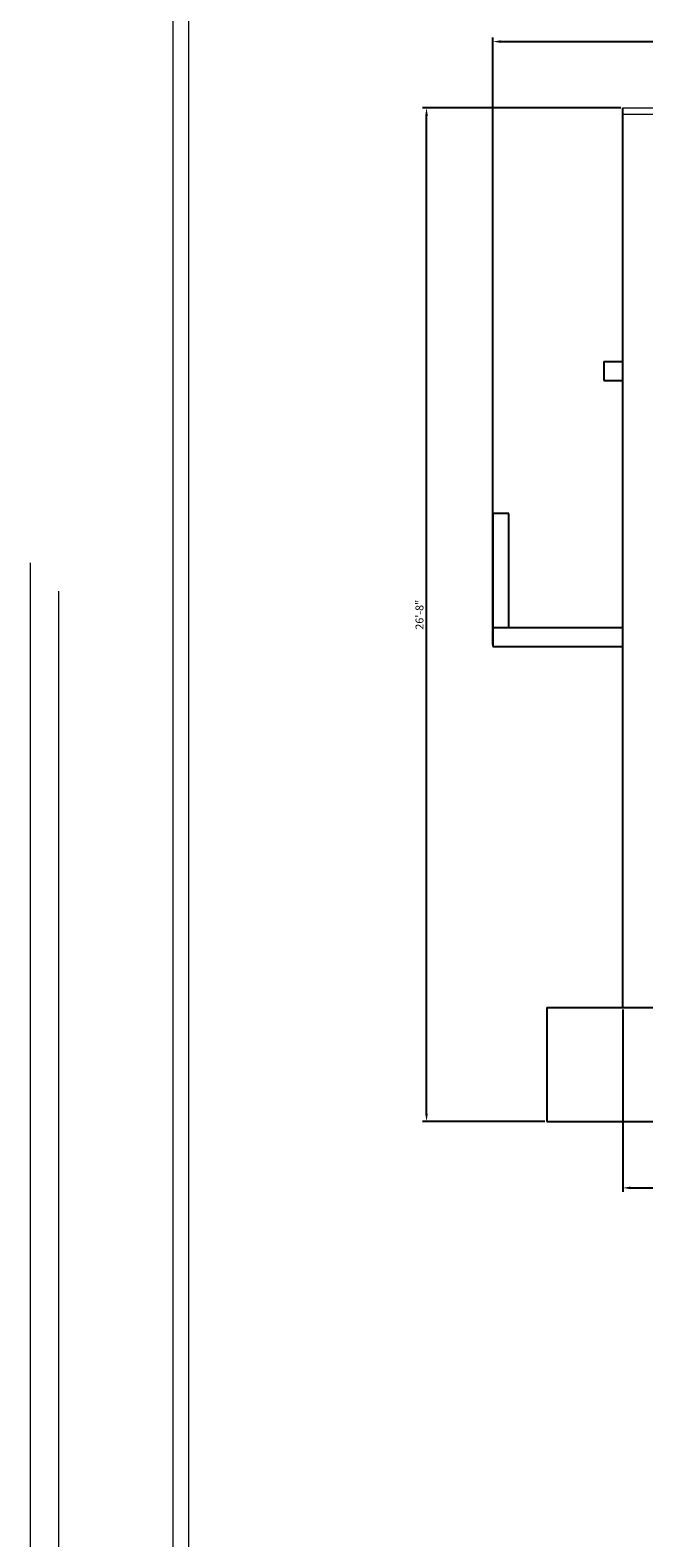
# Model space of a CAD drawing. Units: inches. Extents: x 2443635 to 2446153, y 1826255 to 1827341.
# Tile 15 of 16: x 2445578 to 2445772, y 1826731 to 1827207. Entities that reach past the tile are written whole.
import ezdxf

# ---------------------------------------------------------------- set-up
doc = ezdxf.new("R2010")
doc.units = ezdxf.units.IN
for name, color, linetype, lineweight in [('A-DIMS', 1, 'Continuous', 18), ('A-ELEV', 7, 'Continuous', 25), ('A-ELEV-RAIL', 9, 'Continuous', 18), ('A-REFR', 8, 'Continuous', 13)]:
    doc.layers.add(name, color=color, linetype=linetype, lineweight=lineweight)
doc.styles.get("Standard").update_dxf_attribs({"font": 'arial.ttf'})
doc.dimstyles.new('ISO-25', dxfattribs={"dimtxt": 2.5, "dimasz": 2.5, "dimexe": 1.25, "dimexo": 0.625, "dimtad": 1, "dimlunit": 4, "dimtxsty": 'Standard', "dimcen": 2.5, "dimadec": 0, "dimazin": 0, "dimtfac": 1, "dimtmove": 0, "dimatfit": 3, "dimfxl": 1, "dimarcsym": 0})

# ---------------------------------------------------------------- blocks, each defined once
blk = doc.blocks.new('*D107')
at = {"layer": 'A-DIMS', "color": 0, "lineweight": -2, "transparency": 16777216}
for p, q in [((2445724.56, 1827013.33), (2445724.56, 1827204.9)), ((2446130.56, 1827013.33), (2446130.56, 1827204.9)), ((2445727.06, 1827203.65), (2446128.06, 1827203.65))]:
    blk.add_line(p, q, dxfattribs=at)
at = {"layer": 'A-DIMS', "color": 0, "transparency": 16777216}
for points in [[(2445727.06, 1827204.07), (2445727.06, 1827203.23), (2445724.56, 1827203.65)], [(2446128.06, 1827204.07), (2446128.06, 1827203.23), (2446130.56, 1827203.65)]]:
    blk.add_solid(points, dxfattribs=at)
at = {"layer": 'Defpoints', "color": 0, "transparency": 16777216}
for p in [(2446130.56, 1827203.65), (2445724.56, 1827012.7), (2446130.56, 1827012.7)]:
    blk.add_point(p, dxfattribs=at)
at = {"layer": 'A-DIMS', "color": 0, "transparency": 16777216, "insert": (2445927.56, 1827205.55), "char_height": 2.5, "attachment_point": 5}
blk.add_mtext('33\'-10"', dxfattribs=at)
blk = doc.blocks.new('*D108')
at = {"layer": 'A-DIMS', "color": 0, "lineweight": -2, "transparency": 16777216}
for p, q in [((2445764.93, 1827182.7), (2445702.36, 1827182.7)), ((2445703.61, 1826865.2), (2445703.61, 1827180.2)), ((2445740.93, 1826862.7), (2445702.36, 1826862.7))]:
    blk.add_line(p, q, dxfattribs=at)
at = {"layer": 'A-DIMS', "color": 0, "transparency": 16777216}
for points in [[(2445703.19, 1827180.2), (2445704.03, 1827180.2), (2445703.61, 1827182.7)], [(2445703.19, 1826865.2), (2445704.03, 1826865.2), (2445703.61, 1826862.7)]]:
    blk.add_solid(points, dxfattribs=at)
at = {"layer": 'Defpoints', "color": 0, "transparency": 16777216}
for p in [(2445703.61, 1827182.7), (2445765.56, 1827182.7), (2445741.56, 1826862.7)]:
    blk.add_point(p, dxfattribs=at)
at = {"layer": 'A-DIMS', "color": 0, "transparency": 16777216, "insert": (2445701.71, 1827022.7), "char_height": 2.5, "attachment_point": 5, "rotation": 90}
blk.add_mtext('26\'-8"', dxfattribs=at)
blk = doc.blocks.new('*D109')
at = {"layer": 'A-DIMS', "color": 0, "lineweight": -2, "transparency": 16777216}
for p, q in [((2445765.56, 1826898.08), (2445765.56, 1826840.5)), ((2445906.56, 1826898.08), (2445906.56, 1826840.5)), ((2445768.06, 1826841.75), (2445904.06, 1826841.75))]:
    blk.add_line(p, q, dxfattribs=at)
at = {"layer": 'A-DIMS', "color": 0, "transparency": 16777216}
for points in [[(2445768.06, 1826842.17), (2445768.06, 1826841.33), (2445765.56, 1826841.75)], [(2445904.06, 1826842.17), (2445904.06, 1826841.33), (2445906.56, 1826841.75)]]:
    blk.add_solid(points, dxfattribs=at)
at = {"layer": 'Defpoints', "color": 0, "transparency": 16777216}
for p in [(2445765.56, 1826898.7), (2445906.56, 1826898.7), (2445906.56, 1826841.75)]:
    blk.add_point(p, dxfattribs=at)
at = {"layer": 'A-DIMS', "color": 0, "transparency": 16777216, "insert": (2445836.06, 1826843.65), "char_height": 2.5, "attachment_point": 5}
blk.add_mtext('11\'-9"', dxfattribs=at)
blk = doc.blocks.new('*D111')
at = {"layer": 'A-DIMS', "color": 0, "lineweight": -2, "transparency": 16777216}
for p, q in [((2445816.56, 1826946.08), (2445816.56, 1826840.5)), ((2445765.56, 1826898.08), (2445765.56, 1826840.5)), ((2445768.06, 1826841.75), (2445814.06, 1826841.75))]:
    blk.add_line(p, q, dxfattribs=at)
at = {"layer": 'A-DIMS', "color": 0, "transparency": 16777216}
for points in [[(2445768.06, 1826842.17), (2445768.06, 1826841.33), (2445765.56, 1826841.75)], [(2445814.06, 1826842.17), (2445814.06, 1826841.33), (2445816.56, 1826841.75)]]:
    blk.add_solid(points, dxfattribs=at)
at = {"layer": 'Defpoints', "color": 0, "transparency": 16777216}
for p in [(2445816.56, 1826946.7), (2445765.56, 1826898.7), (2445816.56, 1826841.75)]:
    blk.add_point(p, dxfattribs=at)
at = {"layer": 'A-DIMS', "color": 0, "transparency": 16777216, "insert": (2445791.06, 1826843.65), "char_height": 2.5, "attachment_point": 5}
blk.add_mtext('4\'-3"', dxfattribs=at)

msp = doc.modelspace()

# ---------------------------------------------------------------- linework, layer by layer
at = {"layer": 'A-ELEV'}
for p, q in [((2445765.56, 1826898.701), (2445765.56, 1827182.701)), ((2445724.56, 1827018.701), (2445765.56, 1827018.701)), ((2445741.56, 1826898.701), (2446113.56, 1826898.701)), ((2445741.56, 1826862.701), (2446113.56, 1826862.701))]:
    msp.add_line(p, q, dxfattribs=at)
at = {"layer": 'A-ELEV', "transparency": 33554687}
for p, q in [((2445759.56, 1827102.701), (2445765.56, 1827102.701)), ((2445759.56, 1827102.701), (2445765.56, 1827102.701)), ((2445759.56, 1827102.701), (2445759.56, 1827096.701)), ((2445759.56, 1827096.701), (2445765.56, 1827096.701)), ((2445729.56, 1827054.701), (2445724.56, 1827054.701)), ((2445724.56, 1827054.701), (2445724.56, 1827012.701)), ((2445729.56, 1827018.701), (2445729.56, 1827054.701)), ((2445724.56, 1827012.701), (2445765.56, 1827012.701)), ((2445741.56, 1826898.701), (2445741.56, 1826862.701))]:
    msp.add_line(p, q, dxfattribs=at)
at = {"layer": 'A-ELEV-RAIL', "transparency": 33554687}
for p, q in [((2445765.56, 1827182.701), (2446089.56, 1827182.701)), ((2445765.56, 1827180.701), (2446089.56, 1827180.701))]:
    msp.add_line(p, q, dxfattribs=at)
at = {"layer": 'A-REFR'}
for p, q in [((2445578.466, 1827039.133), (2445578.466, 1826255.288)), ((2445587.466, 1827030.133), (2445587.466, 1826255.288))]:
    msp.add_line(p, q, dxfattribs=at)
at = {"layer": 'A-REFR', "transparency": 33554687}
for p in [(2445623.466, 1827321.207), (2445628.466, 1827316.207)]:
    msp.add_ray(p, (0, -1), dxfattribs=at)

# ---------------------------------------------------------------- dimensions: what is measured, and where the dimension line sits
at = {"layer": 'A-DIMS', "transparency": 33554687}
for base, p1, p2, picture, middle in [((2446130.56, 1827203.651), (2445724.56, 1827012.701), (2446130.56, 1827012.701), '*D107', (2445927.56, 1827205.553)), ((2445816.56, 1826841.751), (2445765.56, 1826898.701), (2445816.56, 1826946.701), '*D111', (2445791.06, 1826843.653)), ((2445906.56, 1826841.751), (2445765.56, 1826898.701), (2445906.56, 1826898.701), '*D109', (2445836.06, 1826843.653))]:
    dim = msp.add_linear_dim(base=base, p1=p1, p2=p2, dimstyle='ISO-25', override={"dimdec": 1, "dimlfac": 1, "dimrnd": 0, "dimzin": 1, "dimdsep": 46, "dimlunit": 4, "dimfrac": 2}, dxfattribs=at)
    dim.commit()
    dim.dimension.update_dxf_attribs({"geometry": picture, "text_midpoint": middle})
dim = msp.add_linear_dim(base=(2445703.61, 1827182.701), p1=(2445741.56, 1826862.701), p2=(2445765.56, 1827182.701), angle=90, dimstyle='ISO-25', override={"dimdec": 1, "dimlfac": 1, "dimrnd": 0, "dimzin": 1, "dimdsep": 46, "dimlunit": 4, "dimfrac": 2}, dxfattribs=at)
dim.commit()
dim.dimension.update_dxf_attribs({"geometry": '*D108', "text_midpoint": (2445701.708, 1827022.701)})

doc.saveas('drawing.dxf')
